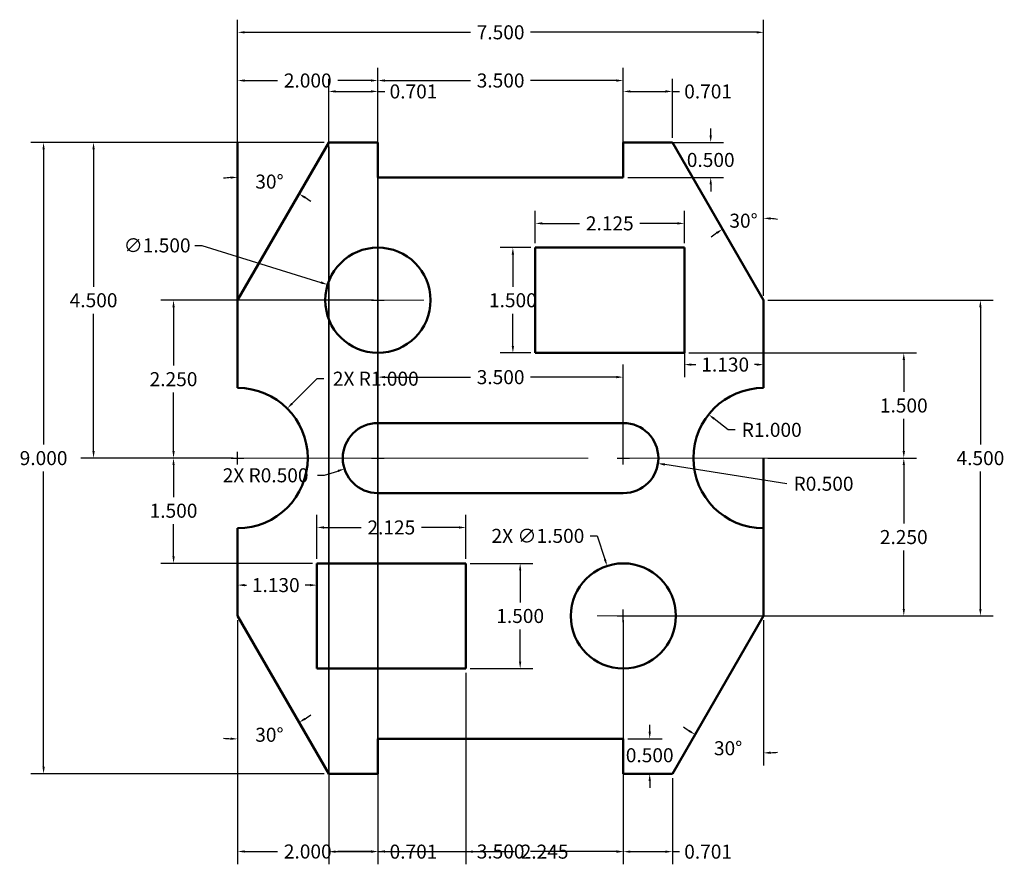
# Model space of a CAD drawing. Units: inches. Extents: x 273.9 to 287.9, y 92.7 to 104.7.
import ezdxf

# ---------------------------------------------------------------- set-up
doc = ezdxf.new("R2010")
doc.units = ezdxf.units.IN
doc.header["$MEASUREMENT"] = 0
doc.linetypes.add('CENTER', pattern=[50.8, 31.75, -6.35, 6.35, -6.35])
for name, color, linetype, lineweight in [('M-CNTR', 114, 'CENTER', 18), ('M-DIMS', 2, 'Continuous', 25), ('M-OUTL', 7, 'Continuous', 50)]:
    doc.layers.add(name, color=color, linetype=linetype, lineweight=lineweight)
doc.styles.get("Standard").update_dxf_attribs({"font": 'arial.ttf'})
doc.dimstyles.get("Standard").update_dxf_attribs({"dimtxt": 0.2, "dimasz": 0.1, "dimexe": 0.18, "dimexo": 0.0625, "dimgap": 0.09, "dimtad": 0, "dimtih": 1, "dimtoh": 1, "dimdec": 3, "dimzin": 0, "dimdsep": 46, "dimtxsty": 'Standard', "dimcen": 0.09, "dimclrd": 1, "dimclre": 1, "dimclrt": 256, "dimadec": 0, "dimazin": 0, "dimtfac": 1, "dimtdec": 3, "dimtofl": 0, "dimtmove": 0, "dimatfit": 3, "dimfxl": 1, "dimtfillclr": 1, "dimtolj": 1, "dimtzin": 0, "dimarcsym": 0})

# ---------------------------------------------------------------- blocks, each defined once
blk = doc.blocks.new('*D1')
at = {"layer": 'Defpoints', "color": 0, "transparency": 16777216}
for p in [(278.973, 94.472), (282.473, 94.472), (282.473, 92.865)]:
    blk.add_point(p, dxfattribs=at)
at = {"layer": 'M-DIMS', "color": 0, "lineweight": -2, "transparency": 16777216}
for p, q in [((278.973, 94.41), (278.973, 92.685)), ((282.473, 94.41), (282.473, 92.685)), ((279.073, 92.865), (280.296, 92.865)), ((282.373, 92.865), (281.15, 92.865))]:
    blk.add_line(p, q, dxfattribs=at)
at = {"layer": 'M-DIMS', "color": 0, "transparency": 16777216}
for points in [[(279.073, 92.882), (279.073, 92.849), (278.973, 92.865)], [(282.373, 92.882), (282.373, 92.849), (282.473, 92.865)]]:
    blk.add_solid(points, dxfattribs=at)
at = {"layer": 'M-DIMS', "color": 0, "transparency": 16777216, "insert": (280.723, 92.865), "char_height": 0.2, "attachment_point": 5}
blk.add_mtext('\\A1;3.500', dxfattribs=at)
blk = doc.blocks.new('*D2')
at = {"layer": 'Defpoints', "color": 0, "transparency": 16777216}
for p in [(282.473, 94.472), (282.473, 93.972), (282.849, 93.972)]:
    blk.add_point(p, dxfattribs=at)
at = {"layer": 'M-DIMS', "color": 0, "lineweight": -2, "transparency": 16777216}
for p, q in [((282.849, 94.572), (282.849, 94.672)), ((282.535, 94.472), (283.029, 94.472)), ((282.535, 93.972), (283.029, 93.972)), ((282.849, 93.872), (282.849, 93.772))]:
    blk.add_line(p, q, dxfattribs=at)
at = {"layer": 'M-DIMS', "color": 0, "transparency": 16777216}
for points in [[(282.833, 94.572), (282.866, 94.572), (282.849, 94.472)], [(282.833, 93.872), (282.866, 93.872), (282.849, 93.972)]]:
    blk.add_solid(points, dxfattribs=at)
at = {"layer": 'M-DIMS', "color": 0, "transparency": 16777216, "insert": (282.849, 94.237), "char_height": 0.2, "attachment_point": 5}
blk.add_mtext('\\A1;0.500', dxfattribs=at)
blk = doc.blocks.new('*D3')
at = {"layer": 'Defpoints', "color": 0, "transparency": 16777216}
for p in [(282.473, 103.854), (278.973, 102.472), (282.473, 102.472)]:
    blk.add_point(p, dxfattribs=at)
at = {"layer": 'M-DIMS', "color": 0, "lineweight": -2, "transparency": 16777216}
for p, q in [((278.973, 102.535), (278.973, 104.034)), ((282.473, 102.535), (282.473, 104.034)), ((279.073, 103.854), (280.296, 103.854)), ((282.373, 103.854), (281.15, 103.854))]:
    blk.add_line(p, q, dxfattribs=at)
at = {"layer": 'M-DIMS', "color": 0, "transparency": 16777216}
for points in [[(279.073, 103.87), (279.073, 103.837), (278.973, 103.854)], [(282.373, 103.87), (282.373, 103.837), (282.473, 103.854)]]:
    blk.add_solid(points, dxfattribs=at)
at = {"layer": 'M-DIMS', "color": 0, "transparency": 16777216, "insert": (280.723, 103.854), "char_height": 0.2, "attachment_point": 5}
blk.add_mtext('\\A1;3.500', dxfattribs=at)
blk = doc.blocks.new('*D4')
at = {"layer": 'Defpoints', "color": 0, "transparency": 16777216}
for p in [(282.473, 99.626), (278.973, 98.472), (282.473, 98.472)]:
    blk.add_point(p, dxfattribs=at)
at = {"layer": 'M-DIMS', "color": 0, "lineweight": -2, "transparency": 16777216}
for p, q in [((278.973, 98.535), (278.973, 99.806)), ((282.473, 98.535), (282.473, 99.806)), ((279.073, 99.626), (280.296, 99.626)), ((282.373, 99.626), (281.15, 99.626))]:
    blk.add_line(p, q, dxfattribs=at)
at = {"layer": 'M-DIMS', "color": 0, "transparency": 16777216}
for points in [[(279.073, 99.643), (279.073, 99.61), (278.973, 99.626)], [(282.373, 99.643), (282.373, 99.61), (282.473, 99.626)]]:
    blk.add_solid(points, dxfattribs=at)
at = {"layer": 'M-DIMS', "color": 0, "transparency": 16777216, "insert": (280.723, 99.626), "char_height": 0.2, "attachment_point": 5}
blk.add_mtext('\\A1;3.500', dxfattribs=at)
blk = doc.blocks.new('*D5')
at = {"layer": 'Defpoints', "color": 0, "transparency": 16777216}
for p in [(280.228, 96.972), (281.002, 96.972), (280.228, 95.472)]:
    blk.add_point(p, dxfattribs=at)
at = {"layer": 'M-DIMS', "color": 0, "lineweight": -2, "transparency": 16777216}
for p, q in [((280.29, 96.972), (281.182, 96.972)), ((281.002, 96.872), (281.002, 96.415)), ((281.002, 95.572), (281.002, 96.03)), ((280.29, 95.472), (281.182, 95.472))]:
    blk.add_line(p, q, dxfattribs=at)
at = {"layer": 'M-DIMS', "color": 0, "transparency": 16777216}
for points in [[(280.985, 96.872), (281.018, 96.872), (281.002, 96.972)], [(280.985, 95.572), (281.018, 95.572), (281.002, 95.472)]]:
    blk.add_solid(points, dxfattribs=at)
at = {"layer": 'M-DIMS', "color": 0, "transparency": 16777216, "insert": (281.002, 96.222), "char_height": 0.2, "attachment_point": 5}
blk.add_mtext('\\A1;1.500', dxfattribs=at)
blk = doc.blocks.new('*D6')
at = {"layer": 'Defpoints', "color": 0, "transparency": 16777216}
for p in [(278.103, 97.484), (278.103, 96.972), (280.228, 96.972)]:
    blk.add_point(p, dxfattribs=at)
at = {"layer": 'M-DIMS', "color": 0, "lineweight": -2, "transparency": 16777216}
for p, q in [((278.103, 97.035), (278.103, 97.664)), ((280.228, 97.035), (280.228, 97.664)), ((278.203, 97.484), (278.735, 97.484)), ((280.128, 97.484), (279.595, 97.484))]:
    blk.add_line(p, q, dxfattribs=at)
at = {"layer": 'M-DIMS', "color": 0, "transparency": 16777216}
for points in [[(278.203, 97.5), (278.203, 97.467), (278.103, 97.484)], [(280.128, 97.5), (280.128, 97.467), (280.228, 97.484)]]:
    blk.add_solid(points, dxfattribs=at)
at = {"layer": 'M-DIMS', "color": 0, "transparency": 16777216, "insert": (279.165, 97.484), "char_height": 0.2, "attachment_point": 5}
blk.add_mtext('\\A1;2.125', dxfattribs=at)
blk = doc.blocks.new('*D7')
at = {"layer": 'Defpoints', "color": 0, "transparency": 16777216}
for p in [(276.973, 97.045), (276.973, 96.662), (278.103, 96.275)]:
    blk.add_point(p, dxfattribs=at)
at = {"layer": 'M-DIMS', "color": 0, "lineweight": -2, "transparency": 16777216}
for p, q in [((276.973, 96.982), (276.973, 96.482)), ((278.103, 96.337), (278.103, 96.842)), ((277.073, 96.662), (277.099, 96.662)), ((278.003, 96.662), (277.935, 96.662))]:
    blk.add_line(p, q, dxfattribs=at)
at = {"layer": 'M-DIMS', "color": 0, "transparency": 16777216}
for points in [[(277.073, 96.678), (277.073, 96.645), (276.973, 96.662)], [(278.003, 96.678), (278.003, 96.645), (278.103, 96.662)]]:
    blk.add_solid(points, dxfattribs=at)
at = {"layer": 'M-DIMS', "color": 0, "transparency": 16777216, "insert": (277.517, 96.662), "char_height": 0.2, "attachment_point": 5}
blk.add_mtext('\\A1;1.130', dxfattribs=at)
blk = doc.blocks.new('*D8')
at = {"layer": 'Defpoints', "color": 0, "transparency": 16777216}
for p in [(276.973, 98.472), (276.059, 96.972), (278.103, 96.972)]:
    blk.add_point(p, dxfattribs=at)
at = {"layer": 'M-DIMS', "color": 0, "lineweight": -2, "transparency": 16777216}
for p, q in [((276.91, 98.472), (275.879, 98.472)), ((276.059, 98.372), (276.059, 97.915)), ((276.059, 97.072), (276.059, 97.53)), ((278.04, 96.972), (275.879, 96.972))]:
    blk.add_line(p, q, dxfattribs=at)
at = {"layer": 'M-DIMS', "color": 0, "transparency": 16777216}
for points in [[(276.043, 98.372), (276.076, 98.372), (276.059, 98.472)], [(276.043, 97.072), (276.076, 97.072), (276.059, 96.972)]]:
    blk.add_solid(points, dxfattribs=at)
at = {"layer": 'M-DIMS', "color": 0, "transparency": 16777216, "insert": (276.059, 97.722), "char_height": 0.2, "attachment_point": 5}
blk.add_mtext('\\A1;1.500', dxfattribs=at)
blk = doc.blocks.new('*D9')
at = {"layer": 'Defpoints', "color": 0, "transparency": 16777216}
for p in [(278.973, 100.722), (276.059, 98.472), (276.973, 98.472)]:
    blk.add_point(p, dxfattribs=at)
at = {"layer": 'M-DIMS', "color": 0, "lineweight": -2, "transparency": 16777216}
for p, q in [((278.91, 100.722), (275.879, 100.722)), ((276.059, 100.622), (276.059, 99.79)), ((276.059, 98.572), (276.059, 99.405)), ((276.91, 98.472), (275.879, 98.472))]:
    blk.add_line(p, q, dxfattribs=at)
at = {"layer": 'M-DIMS', "color": 0, "transparency": 16777216}
for points in [[(276.043, 100.622), (276.076, 100.622), (276.059, 100.722)], [(276.043, 98.572), (276.076, 98.572), (276.059, 98.472)]]:
    blk.add_solid(points, dxfattribs=at)
at = {"layer": 'M-DIMS', "color": 0, "transparency": 16777216, "insert": (276.059, 99.597), "char_height": 0.2, "attachment_point": 5}
blk.add_mtext('\\A1;2.250', dxfattribs=at)
blk = doc.blocks.new('*D10')
at = {"layer": 'Defpoints', "color": 0, "transparency": 16777216}
for p in [(281.218, 101.818), (281.218, 101.472), (283.343, 101.472)]:
    blk.add_point(p, dxfattribs=at)
at = {"layer": 'M-DIMS', "color": 0, "lineweight": -2, "transparency": 16777216}
for p, q in [((281.218, 101.535), (281.218, 101.998)), ((283.343, 101.535), (283.343, 101.998)), ((281.318, 101.818), (281.85, 101.818)), ((283.243, 101.818), (282.71, 101.818))]:
    blk.add_line(p, q, dxfattribs=at)
at = {"layer": 'M-DIMS', "color": 0, "transparency": 16777216}
for points in [[(281.318, 101.834), (281.318, 101.801), (281.218, 101.818)], [(283.243, 101.834), (283.243, 101.801), (283.343, 101.818)]]:
    blk.add_solid(points, dxfattribs=at)
at = {"layer": 'M-DIMS', "color": 0, "transparency": 16777216, "insert": (282.28, 101.818), "char_height": 0.2, "attachment_point": 5}
blk.add_mtext('\\A1;2.125', dxfattribs=at)
blk = doc.blocks.new('*D11')
at = {"layer": 'Defpoints', "color": 0, "transparency": 16777216}
for p in [(281.218, 101.472), (280.898, 99.972), (281.218, 99.972)]:
    blk.add_point(p, dxfattribs=at)
at = {"layer": 'M-DIMS', "color": 0, "lineweight": -2, "transparency": 16777216}
for p, q in [((281.155, 101.472), (280.718, 101.472)), ((280.898, 101.372), (280.898, 100.915)), ((280.898, 100.072), (280.898, 100.53)), ((281.155, 99.972), (280.718, 99.972))]:
    blk.add_line(p, q, dxfattribs=at)
at = {"layer": 'M-DIMS', "color": 0, "transparency": 16777216}
for points in [[(280.881, 101.372), (280.915, 101.372), (280.898, 101.472)], [(280.881, 100.072), (280.915, 100.072), (280.898, 99.972)]]:
    blk.add_solid(points, dxfattribs=at)
at = {"layer": 'M-DIMS', "color": 0, "transparency": 16777216, "insert": (280.898, 100.722), "char_height": 0.2, "attachment_point": 5}
blk.add_mtext('\\A1;1.500', dxfattribs=at)
blk = doc.blocks.new('*D12')
at = {"layer": 'Defpoints', "color": 0, "transparency": 16777216}
for p in [(283.343, 100.363), (284.473, 99.805), (284.473, 99.79)]:
    blk.add_point(p, dxfattribs=at)
at = {"layer": 'M-DIMS', "color": 0, "lineweight": -2, "transparency": 16777216}
for p, q in [((283.343, 100.3), (283.343, 99.625)), ((284.473, 99.853), (284.473, 99.985)), ((283.443, 99.805), (283.508, 99.805)), ((284.373, 99.805), (284.343, 99.805))]:
    blk.add_line(p, q, dxfattribs=at)
at = {"layer": 'M-DIMS', "color": 0, "transparency": 16777216}
for points in [[(283.443, 99.821), (283.443, 99.788), (283.343, 99.805)], [(284.373, 99.821), (284.373, 99.788), (284.473, 99.805)]]:
    blk.add_solid(points, dxfattribs=at)
at = {"layer": 'M-DIMS', "color": 0, "transparency": 16777216, "insert": (283.926, 99.805), "char_height": 0.2, "attachment_point": 5}
blk.add_mtext('\\A1;1.130', dxfattribs=at)
blk = doc.blocks.new('*D13')
at = {"layer": 'Defpoints', "color": 0, "transparency": 16777216}
for p in [(283.174, 102.972), (284.073, 101.821), (284.473, 100.722), (284.473, 100.722), (284.473, 99.472)]:
    blk.add_point(p, dxfattribs=at)
at = {"layer": 'M-DIMS', "color": 0, "lineweight": -2, "transparency": 16777216}
blk.add_line((284.473, 100.785), (284.473, 102.071), dxfattribs=at)
for start, end in [(80.1925, 85.0963), (124.9037, 129.8075)]:
    blk.add_arc((284.473, 100.722), 1.169, start, end, dxfattribs=at)
at = {"layer": 'M-DIMS', "color": 0, "transparency": 16777216}
for points in [[(284.572, 101.87), (284.573, 101.904), (284.473, 101.891)], [(283.795, 101.695), (283.813, 101.667), (283.888, 101.735)]]:
    blk.add_solid(points, dxfattribs=at)
at = {"layer": 'M-DIMS', "color": 0, "transparency": 16777216, "insert": (284.187, 101.856), "char_height": 0.2, "attachment_point": 5}
blk.add_mtext('\\A1;30°', dxfattribs=at)
blk = doc.blocks.new('*D14')
at = {"layer": 'Defpoints', "color": 0, "transparency": 16777216}
for p in [(276.973, 96.222), (276.973, 96.222), (277.277, 94.496), (276.973, 94.41), (278.272, 93.972)]:
    blk.add_point(p, dxfattribs=at)
at = {"layer": 'M-DIMS', "color": 0, "lineweight": -2, "transparency": 16777216}
for start, end in [(303.2689, 306.5377), (263.4623, 266.7311)]:
    blk.add_arc((276.973, 96.222), 1.753, start, end, dxfattribs=at)
at = {"layer": 'M-DIMS', "color": 0, "transparency": 16777216}
for points in [[(277.943, 94.743), (277.925, 94.771), (277.849, 94.704)], [(276.873, 94.489), (276.872, 94.456), (276.973, 94.469)]]:
    blk.add_solid(points, dxfattribs=at)
at = {"layer": 'M-DIMS', "color": 0, "transparency": 16777216, "insert": (277.426, 94.529), "char_height": 0.2, "attachment_point": 5}
blk.add_mtext('\\A1;30°', dxfattribs=at)
blk = doc.blocks.new('*D15')
at = {"layer": 'Defpoints', "color": 0, "transparency": 16777216}
for p in [(276.973, 96.222), (278.973, 93.972), (278.973, 92.865)]:
    blk.add_point(p, dxfattribs=at)
at = {"layer": 'M-DIMS', "color": 0, "lineweight": -2, "transparency": 16777216}
for p, q in [((276.973, 96.16), (276.973, 92.685)), ((278.973, 93.91), (278.973, 92.685)), ((277.073, 92.865), (277.544, 92.865)), ((278.873, 92.865), (278.401, 92.865))]:
    blk.add_line(p, q, dxfattribs=at)
at = {"layer": 'M-DIMS', "color": 0, "transparency": 16777216}
for points in [[(277.073, 92.882), (277.073, 92.849), (276.973, 92.865)], [(278.873, 92.882), (278.873, 92.849), (278.973, 92.865)]]:
    blk.add_solid(points, dxfattribs=at)
at = {"layer": 'M-DIMS', "color": 0, "transparency": 16777216, "insert": (277.973, 92.865), "char_height": 0.2, "attachment_point": 5}
blk.add_mtext('\\A1;2.000', dxfattribs=at)
blk = doc.blocks.new('*D16')
at = {"layer": 'Defpoints', "color": 0, "transparency": 16777216}
for p in [(283.69, 99.094), (284.473, 98.472)]:
    blk.add_point(p, dxfattribs=at)
at = {"layer": 'M-DIMS', "color": 0, "lineweight": -2, "transparency": 16777216}
for p, q in [((283.966, 98.875), (283.768, 99.032)), ((284.066, 98.875), (283.966, 98.875))]:
    blk.add_line(p, q, dxfattribs=at)
at = {"layer": 'M-DIMS', "color": 0, "transparency": 16777216}
blk.add_solid([(283.778, 99.045), (283.758, 99.019), (283.69, 99.094)], dxfattribs=at)
at = {"layer": 'M-DIMS', "color": 0, "transparency": 16777216, "insert": (284.589, 98.875), "char_height": 0.2, "attachment_point": 5}
blk.add_mtext('\\A1;R1.000', dxfattribs=at)
blk = doc.blocks.new('*D17')
at = {"layer": 'Defpoints', "color": 0, "transparency": 16777216}
for p in [(282.473, 98.472), (282.967, 98.395)]:
    blk.add_point(p, dxfattribs=at)
at = {"layer": 'M-DIMS', "color": 0, "lineweight": -2, "transparency": 16777216}
for p, q in [((282.473, 98.382), (282.473, 98.562)), ((282.383, 98.472), (282.563, 98.472)), ((284.805, 98.107), (283.065, 98.38))]:
    blk.add_line(p, q, dxfattribs=at)
at = {"layer": 'M-DIMS', "color": 0, "transparency": 16777216}
blk.add_solid([(283.068, 98.396), (283.063, 98.363), (282.967, 98.395)], dxfattribs=at)
at = {"layer": 'M-DIMS', "color": 0, "transparency": 16777216, "insert": (285.328, 98.107), "char_height": 0.2, "attachment_point": 5}
blk.add_mtext('\\A1;R0.500', dxfattribs=at)
blk = doc.blocks.new('*D18')
at = {"layer": 'Defpoints', "color": 0, "transparency": 16777216}
for p in [(284.473, 98.472), (282.473, 96.222), (286.472, 96.222)]:
    blk.add_point(p, dxfattribs=at)
at = {"layer": 'M-DIMS', "color": 0, "lineweight": -2, "transparency": 16777216}
for p, q in [((284.535, 98.472), (286.652, 98.472)), ((286.472, 98.372), (286.472, 97.54)), ((286.472, 96.322), (286.472, 97.155)), ((282.535, 96.222), (286.652, 96.222))]:
    blk.add_line(p, q, dxfattribs=at)
at = {"layer": 'M-DIMS', "color": 0, "transparency": 16777216}
for points in [[(286.456, 98.372), (286.489, 98.372), (286.472, 98.472)], [(286.456, 96.322), (286.489, 96.322), (286.472, 96.222)]]:
    blk.add_solid(points, dxfattribs=at)
at = {"layer": 'M-DIMS', "color": 0, "transparency": 16777216, "insert": (286.472, 97.347), "char_height": 0.2, "attachment_point": 5}
blk.add_mtext('\\A1;2.250', dxfattribs=at)
blk = doc.blocks.new('*D19')
at = {"layer": 'Defpoints', "color": 0, "transparency": 16777216}
for p in [(283.343, 99.972), (286.472, 99.972), (284.473, 98.472)]:
    blk.add_point(p, dxfattribs=at)
at = {"layer": 'M-DIMS', "color": 0, "lineweight": -2, "transparency": 16777216}
for p, q in [((283.405, 99.972), (286.652, 99.972)), ((286.472, 99.872), (286.472, 99.415)), ((286.472, 98.572), (286.472, 99.03)), ((284.535, 98.472), (286.652, 98.472))]:
    blk.add_line(p, q, dxfattribs=at)
at = {"layer": 'M-DIMS', "color": 0, "transparency": 16777216}
for points in [[(286.456, 99.872), (286.489, 99.872), (286.472, 99.972)], [(286.456, 98.572), (286.489, 98.572), (286.472, 98.472)]]:
    blk.add_solid(points, dxfattribs=at)
at = {"layer": 'M-DIMS', "color": 0, "transparency": 16777216, "insert": (286.472, 99.222), "char_height": 0.2, "attachment_point": 5}
blk.add_mtext('\\A1;1.500', dxfattribs=at)
blk = doc.blocks.new('*D20')
at = {"layer": 'Defpoints', "color": 0, "transparency": 16777216}
for p in [(284.473, 100.722), (287.565, 100.722), (284.473, 96.222)]:
    blk.add_point(p, dxfattribs=at)
at = {"layer": 'M-DIMS', "color": 0, "lineweight": -2, "transparency": 16777216}
for p, q in [((284.535, 100.722), (287.745, 100.722)), ((287.565, 100.622), (287.565, 98.665)), ((287.565, 96.322), (287.565, 98.28)), ((284.535, 96.222), (287.745, 96.222))]:
    blk.add_line(p, q, dxfattribs=at)
at = {"layer": 'M-DIMS', "color": 0, "transparency": 16777216}
for points in [[(287.548, 100.622), (287.581, 100.622), (287.565, 100.722)], [(287.548, 96.322), (287.581, 96.322), (287.565, 96.222)]]:
    blk.add_solid(points, dxfattribs=at)
at = {"layer": 'M-DIMS', "color": 0, "transparency": 16777216, "insert": (287.565, 98.472), "char_height": 0.2, "attachment_point": 5}
blk.add_mtext('\\A1;4.500', dxfattribs=at)
blk = doc.blocks.new('*D21')
at = {"layer": 'Defpoints', "color": 0, "transparency": 16777216}
for p in [(276.973, 102.972), (278.272, 102.972), (277.277, 102.447), (276.973, 100.722), (276.973, 99.472)]:
    blk.add_point(p, dxfattribs=at)
at = {"layer": 'M-DIMS', "color": 0, "lineweight": -2, "transparency": 16777216}
for start, end in [(93.2724, 96.5449), (53.4551, 56.7276)]:
    blk.add_arc((276.973, 100.722), 1.751, start, end, dxfattribs=at)
at = {"layer": 'M-DIMS', "color": 0, "transparency": 16777216}
for points in [[(276.872, 102.487), (276.873, 102.454), (276.973, 102.474)], [(277.925, 102.172), (277.942, 102.201), (277.848, 102.239)]]:
    blk.add_solid(points, dxfattribs=at)
at = {"layer": 'M-DIMS', "color": 0, "transparency": 16777216, "insert": (277.427, 102.413), "char_height": 0.2, "attachment_point": 5}
blk.add_mtext('\\A1;30°', dxfattribs=at)
blk = doc.blocks.new('*D22')
at = {"layer": 'Defpoints', "color": 0, "transparency": 16777216}
for p in [(284.473, 104.541), (276.973, 100.722), (284.473, 100.722)]:
    blk.add_point(p, dxfattribs=at)
at = {"layer": 'M-DIMS', "color": 0, "lineweight": -2, "transparency": 16777216}
for p, q in [((276.973, 100.785), (276.973, 104.721)), ((284.473, 100.785), (284.473, 104.721)), ((277.073, 104.541), (280.296, 104.541)), ((284.373, 104.541), (281.149, 104.541))]:
    blk.add_line(p, q, dxfattribs=at)
at = {"layer": 'M-DIMS', "color": 0, "transparency": 16777216}
for points in [[(277.073, 104.557), (277.073, 104.524), (276.973, 104.541)], [(284.373, 104.557), (284.373, 104.524), (284.473, 104.541)]]:
    blk.add_solid(points, dxfattribs=at)
at = {"layer": 'M-DIMS', "color": 0, "transparency": 16777216, "insert": (280.723, 104.541), "char_height": 0.2, "attachment_point": 5}
blk.add_mtext('\\A1;7.500', dxfattribs=at)
blk = doc.blocks.new('*D23')
at = {"layer": 'Defpoints', "color": 0, "transparency": 16777216}
for p in [(278.973, 103.854), (278.973, 102.972), (276.973, 100.722)]:
    blk.add_point(p, dxfattribs=at)
at = {"layer": 'M-DIMS', "color": 0, "lineweight": -2, "transparency": 16777216}
for p, q in [((276.973, 100.785), (276.973, 104.034)), ((278.973, 103.035), (278.973, 104.034)), ((277.073, 103.854), (277.544, 103.854)), ((278.873, 103.854), (278.401, 103.854))]:
    blk.add_line(p, q, dxfattribs=at)
at = {"layer": 'M-DIMS', "color": 0, "transparency": 16777216}
for points in [[(277.073, 103.87), (277.073, 103.837), (276.973, 103.854)], [(278.873, 103.87), (278.873, 103.837), (278.973, 103.854)]]:
    blk.add_solid(points, dxfattribs=at)
at = {"layer": 'M-DIMS', "color": 0, "transparency": 16777216, "insert": (277.973, 103.854), "char_height": 0.2, "attachment_point": 5}
blk.add_mtext('\\A1;2.000', dxfattribs=at)
blk = doc.blocks.new('*D24')
at = {"layer": 'Defpoints', "color": 0, "transparency": 16777216}
for p in [(282.473, 102.972), (283.719, 102.972), (282.473, 102.472)]:
    blk.add_point(p, dxfattribs=at)
at = {"layer": 'M-DIMS', "color": 0, "lineweight": -2, "transparency": 16777216}
for p, q in [((283.719, 103.072), (283.719, 103.172)), ((282.535, 102.972), (283.899, 102.972)), ((282.535, 102.472), (283.899, 102.472)), ((283.719, 102.372), (283.719, 102.272))]:
    blk.add_line(p, q, dxfattribs=at)
at = {"layer": 'M-DIMS', "color": 0, "transparency": 16777216}
for points in [[(283.702, 103.072), (283.736, 103.072), (283.719, 102.972)], [(283.702, 102.372), (283.736, 102.372), (283.719, 102.472)]]:
    blk.add_solid(points, dxfattribs=at)
at = {"layer": 'M-DIMS', "color": 0, "transparency": 16777216, "insert": (283.719, 102.722), "char_height": 0.2, "attachment_point": 5}
blk.add_mtext('\\A1;0.500', dxfattribs=at)
blk = doc.blocks.new('*D25')
at = {"layer": 'Defpoints', "color": 0, "transparency": 16777216}
for p in [(278.256, 100.945), (279.689, 100.5)]:
    blk.add_point(p, dxfattribs=at)
at = {"layer": 'M-DIMS', "color": 0, "lineweight": -2, "transparency": 16777216}
for p, q in [((276.361, 101.504), (276.461, 101.504)), ((276.461, 101.504), (278.161, 100.975)), ((278.973, 100.632), (278.973, 100.812)), ((278.883, 100.722), (279.063, 100.722))]:
    blk.add_line(p, q, dxfattribs=at)
at = {"layer": 'M-DIMS', "color": 0, "transparency": 16777216}
blk.add_solid([(278.166, 100.991), (278.156, 100.959), (278.256, 100.945)], dxfattribs=at)
at = {"layer": 'M-DIMS', "color": 0, "transparency": 16777216, "insert": (275.825, 101.504), "char_height": 0.2, "attachment_point": 5}
blk.add_mtext('\\A1;∅1.500', dxfattribs=at)
blk = doc.blocks.new('*D26')
at = {"layer": 'Defpoints', "color": 0, "transparency": 16777216}
for p in [(278.272, 102.972), (274.206, 93.972), (278.272, 93.972)]:
    blk.add_point(p, dxfattribs=at)
at = {"layer": 'M-DIMS', "color": 0, "lineweight": -2, "transparency": 16777216}
for p, q in [((278.209, 102.972), (274.026, 102.972)), ((274.206, 102.872), (274.206, 98.665)), ((274.206, 94.072), (274.206, 98.28)), ((278.209, 93.972), (274.026, 93.972))]:
    blk.add_line(p, q, dxfattribs=at)
at = {"layer": 'M-DIMS', "color": 0, "transparency": 16777216}
for points in [[(274.19, 102.872), (274.223, 102.872), (274.206, 102.972)], [(274.19, 94.072), (274.223, 94.072), (274.206, 93.972)]]:
    blk.add_solid(points, dxfattribs=at)
at = {"layer": 'M-DIMS', "color": 0, "transparency": 16777216, "insert": (274.206, 98.472), "char_height": 0.2, "attachment_point": 5}
blk.add_mtext('\\A1;9.000', dxfattribs=at)
blk = doc.blocks.new('*D27')
at = {"layer": 'Defpoints', "color": 0, "transparency": 16777216}
for p in [(278.272, 102.972), (274.919, 98.472), (276.973, 98.472)]:
    blk.add_point(p, dxfattribs=at)
at = {"layer": 'M-DIMS', "color": 0, "lineweight": -2, "transparency": 16777216}
for p, q in [((278.209, 102.972), (274.739, 102.972)), ((274.919, 102.872), (274.919, 100.915)), ((274.919, 98.572), (274.919, 100.53)), ((276.91, 98.472), (274.739, 98.472))]:
    blk.add_line(p, q, dxfattribs=at)
at = {"layer": 'M-DIMS', "color": 0, "transparency": 16777216}
for points in [[(274.902, 102.872), (274.935, 102.872), (274.919, 102.972)], [(274.902, 98.572), (274.935, 98.572), (274.919, 98.472)]]:
    blk.add_solid(points, dxfattribs=at)
at = {"layer": 'M-DIMS', "color": 0, "transparency": 16777216, "insert": (274.919, 100.722), "char_height": 0.2, "attachment_point": 5}
blk.add_mtext('\\A1;4.500', dxfattribs=at)
blk = doc.blocks.new('*D28')
at = {"layer": 'Defpoints', "color": 0, "transparency": 16777216}
for p in [(284.473, 98.472), (284.473, 96.222), (284.473, 96.222), (283.805, 94.388), (283.174, 93.972)]:
    blk.add_point(p, dxfattribs=at)
at = {"layer": 'M-DIMS', "color": 0, "lineweight": -2, "transparency": 16777216}
blk.add_line((284.473, 96.16), (284.473, 94.09), dxfattribs=at)
for start, end in [(234.1288, 237.0644), (272.9356, 275.8712)]:
    blk.add_arc((284.473, 96.222), 1.952, start, end, dxfattribs=at)
at = {"layer": 'M-DIMS', "color": 0, "transparency": 16777216}
for points in [[(283.42, 94.598), (283.403, 94.57), (283.497, 94.532)], [(284.573, 94.256), (284.572, 94.29), (284.473, 94.27)]]:
    blk.add_solid(points, dxfattribs=at)
at = {"layer": 'M-DIMS', "color": 0, "transparency": 16777216, "insert": (283.967, 94.337), "char_height": 0.2, "attachment_point": 5}
blk.add_mtext('\\A1;30°', dxfattribs=at)
blk = doc.blocks.new('CUTOUT-RECT-2.125X1.50')
for p, q in [((0, 1.5), (0, 0)), ((2.125, 1.5), (0, 1.5)), ((2.125, 0), (2.125, 1.5)), ((0, 0), (2.125, 0))]:
    blk.add_line(p, q)
blk = doc.blocks.new('HOLE-DIA-1.50')
blk.add_circle((0.75, 0.75), 0.75)
blk = doc.blocks.new('*D31')
at = {"layer": 'Defpoints', "color": 0, "transparency": 16777216}
for p in [(278.973, 103.698), (278.272, 93.972), (278.973, 93.972)]:
    blk.add_point(p, dxfattribs=at)
at = {"layer": 'M-DIMS', "color": 1, "lineweight": -2, "transparency": 16777216}
for p, q in [((278.272, 94.035), (278.272, 103.878)), ((278.973, 94.035), (278.973, 103.878)), ((278.372, 103.698), (278.873, 103.698)), ((278.973, 103.698), (279.073, 103.698))]:
    blk.add_line(p, q, dxfattribs=at)
at = {"layer": 'M-DIMS', "color": 1, "transparency": 16777216}
for points in [[(278.372, 103.715), (278.372, 103.682), (278.272, 103.698)], [(278.873, 103.715), (278.873, 103.682), (278.973, 103.698)]]:
    blk.add_solid(points, dxfattribs=at)
at = {"layer": 'M-DIMS', "transparency": 16777216, "insert": (279.481, 103.698), "char_height": 0.2, "attachment_point": 5}
blk.add_mtext('\\A1;0.701', dxfattribs=at)
blk = doc.blocks.new('*D32')
at = {"layer": 'Defpoints', "color": 0, "transparency": 16777216}
for p in [(282.473, 96.222), (280.228, 95.472), (282.473, 92.863)]:
    blk.add_point(p, dxfattribs=at)
at = {"layer": 'M-DIMS', "color": 1, "lineweight": -2, "transparency": 16777216}
for p, q in [((282.473, 96.16), (282.473, 92.683)), ((280.228, 95.41), (280.228, 92.683)), ((280.328, 92.863), (280.92, 92.863)), ((282.373, 92.863), (281.78, 92.863))]:
    blk.add_line(p, q, dxfattribs=at)
at = {"layer": 'M-DIMS', "color": 1, "transparency": 16777216}
for points in [[(280.328, 92.879), (280.328, 92.846), (280.228, 92.863)], [(282.373, 92.879), (282.373, 92.846), (282.473, 92.863)]]:
    blk.add_solid(points, dxfattribs=at)
at = {"layer": 'M-DIMS', "transparency": 16777216, "insert": (281.35, 92.863), "char_height": 0.2, "attachment_point": 5}
blk.add_mtext('\\A1;2.245', dxfattribs=at)
blk = doc.blocks.new('*D33')
at = {"layer": 'Defpoints', "color": 0, "transparency": 16777216}
for p in [(278.272, 102.972), (278.973, 102.972), (278.973, 92.863)]:
    blk.add_point(p, dxfattribs=at)
at = {"layer": 'M-DIMS', "color": 1, "lineweight": -2, "transparency": 16777216}
for p, q in [((278.272, 102.91), (278.272, 92.683)), ((278.973, 102.91), (278.973, 92.683)), ((278.372, 92.863), (278.873, 92.863)), ((278.973, 92.863), (279.073, 92.863))]:
    blk.add_line(p, q, dxfattribs=at)
at = {"layer": 'M-DIMS', "color": 1, "transparency": 16777216}
for points in [[(278.372, 92.879), (278.372, 92.846), (278.272, 92.863)], [(278.873, 92.879), (278.873, 92.846), (278.973, 92.863)]]:
    blk.add_solid(points, dxfattribs=at)
at = {"layer": 'M-DIMS', "transparency": 16777216, "insert": (279.481, 92.863), "char_height": 0.2, "attachment_point": 5}
blk.add_mtext('\\A1;0.701', dxfattribs=at)
blk = doc.blocks.new('*D34')
at = {"layer": 'Defpoints', "color": 0, "transparency": 16777216}
for p in [(283.174, 103.698), (282.473, 102.972), (283.174, 102.972)]:
    blk.add_point(p, dxfattribs=at)
at = {"layer": 'M-DIMS', "color": 1, "lineweight": -2, "transparency": 16777216}
for p, q in [((282.473, 103.035), (282.473, 103.878)), ((283.174, 103.035), (283.174, 103.878)), ((282.573, 103.698), (283.074, 103.698)), ((283.174, 103.698), (283.274, 103.698))]:
    blk.add_line(p, q, dxfattribs=at)
at = {"layer": 'M-DIMS', "color": 1, "transparency": 16777216}
for points in [[(282.573, 103.715), (282.573, 103.682), (282.473, 103.698)], [(283.074, 103.715), (283.074, 103.682), (283.174, 103.698)]]:
    blk.add_solid(points, dxfattribs=at)
at = {"layer": 'M-DIMS', "transparency": 16777216, "insert": (283.682, 103.698), "char_height": 0.2, "attachment_point": 5}
blk.add_mtext('\\A1;0.701', dxfattribs=at)
blk = doc.blocks.new('*D35')
at = {"layer": 'Defpoints', "color": 0, "transparency": 16777216}
for p in [(282.473, 93.972), (283.174, 93.972), (283.174, 92.863)]:
    blk.add_point(p, dxfattribs=at)
at = {"layer": 'M-DIMS', "color": 1, "lineweight": -2, "transparency": 16777216}
for p, q in [((282.473, 93.91), (282.473, 92.683)), ((283.174, 93.91), (283.174, 92.683)), ((282.573, 92.863), (283.074, 92.863)), ((283.174, 92.863), (283.274, 92.863))]:
    blk.add_line(p, q, dxfattribs=at)
at = {"layer": 'M-DIMS', "color": 1, "transparency": 16777216}
for points in [[(282.573, 92.879), (282.573, 92.846), (282.473, 92.863)], [(283.074, 92.879), (283.074, 92.846), (283.174, 92.863)]]:
    blk.add_solid(points, dxfattribs=at)
at = {"layer": 'M-DIMS', "transparency": 16777216, "insert": (283.682, 92.863), "char_height": 0.2, "attachment_point": 5}
blk.add_mtext('\\A1;0.701', dxfattribs=at)
blk = doc.blocks.new('*D36')
at = {"layer": 'Defpoints', "color": 0, "transparency": 16777216}
for p in [(277.68, 99.18), (276.973, 98.472)]:
    blk.add_point(p, dxfattribs=at)
at = {"layer": 'M-DIMS', "color": 1, "lineweight": -2, "transparency": 16777216}
for p, q in [((278.104, 99.604), (277.75, 99.25)), ((278.204, 99.604), (278.104, 99.604)), ((276.973, 98.382), (276.973, 98.562)), ((276.883, 98.472), (277.063, 98.472))]:
    blk.add_line(p, q, dxfattribs=at)
at = {"layer": 'M-DIMS', "color": 1, "transparency": 16777216}
blk.add_solid([(277.739, 99.262), (277.762, 99.239), (277.68, 99.18)], dxfattribs=at)
at = {"layer": 'M-DIMS', "transparency": 16777216, "insert": (278.943, 99.604), "char_height": 0.2, "attachment_point": 5}
blk.add_mtext('\\A1;2X R1.000', dxfattribs=at)
blk = doc.blocks.new('*D37')
at = {"layer": 'Defpoints', "color": 0, "transparency": 16777216}
for p in [(278.973, 98.472), (278.497, 98.319)]:
    blk.add_point(p, dxfattribs=at)
at = {"layer": 'M-DIMS', "color": 1, "lineweight": -2, "transparency": 16777216}
for p, q in [((278.973, 98.382), (278.973, 98.562)), ((278.883, 98.472), (279.063, 98.472)), ((278.211, 98.227), (278.402, 98.288)), ((278.111, 98.227), (278.211, 98.227))]:
    blk.add_line(p, q, dxfattribs=at)
at = {"layer": 'M-DIMS', "color": 1, "transparency": 16777216}
blk.add_solid([(278.396, 98.304), (278.407, 98.272), (278.497, 98.319)], dxfattribs=at)
at = {"layer": 'M-DIMS', "transparency": 16777216, "insert": (277.372, 98.227), "char_height": 0.2, "attachment_point": 5}
blk.add_mtext('\\A1;2X R0.500', dxfattribs=at)
blk = doc.blocks.new('*D38')
at = {"layer": 'Defpoints', "color": 0, "transparency": 16777216}
for p in [(282.241, 96.936), (282.704, 95.509)]:
    blk.add_point(p, dxfattribs=at)
at = {"layer": 'M-DIMS', "color": 1, "lineweight": -2, "transparency": 16777216}
for p, q in [((282.002, 97.364), (282.102, 97.364)), ((282.102, 97.364), (282.21, 97.031)), ((282.383, 96.222), (282.563, 96.222)), ((282.473, 96.132), (282.473, 96.312))]:
    blk.add_line(p, q, dxfattribs=at)
at = {"layer": 'M-DIMS', "color": 1, "transparency": 16777216}
blk.add_solid([(282.226, 97.036), (282.194, 97.026), (282.241, 96.936)], dxfattribs=at)
at = {"layer": 'M-DIMS', "transparency": 16777216, "insert": (281.255, 97.364), "char_height": 0.2, "attachment_point": 5}
blk.add_mtext('\\A1;2X ∅1.500', dxfattribs=at)

msp = doc.modelspace()

# ---------------------------------------------------------------- linework, layer by layer
at = {"layer": 'M-CNTR'}
for p, q in [((278.9726, 101.4724), (278.9726, 93.5887)), ((276.9726, 100.7224), (279.6282, 100.7224)), ((276.2737, 98.4724), (281.9726, 98.4724)), ((282.4726, 98.4724), (285.2073, 98.4724)), ((284.4726, 96.2224), (282.0977, 96.2224))]:
    msp.add_line(p, q, dxfattribs=at)
at = {"layer": 'M-OUTL'}
for p, q in [((276.9726, 99.4724), (276.9726, 102.9724)), ((276.9726, 100.7224), (278.2716, 102.9724)), ((278.2716, 102.9724), (278.9726, 102.9724)), ((278.9726, 102.9724), (278.9726, 102.4724)), ((282.4726, 102.4724), (282.4726, 102.9724)), ((282.4726, 102.9724), (283.1735, 102.9724)), ((284.4726, 100.7224), (283.1735, 102.9724)), ((278.9726, 102.4724), (282.4726, 102.4724)), ((284.4726, 99.4724), (284.4726, 100.7224)), ((278.9726, 98.9724), (282.4726, 98.9724)), ((284.4726, 98.4724), (284.4726, 96.2224)), ((278.9726, 97.9724), (282.4726, 97.9724)), ((276.9726, 96.2224), (276.9726, 97.4724)), ((276.9726, 96.2224), (278.2716, 93.9724)), ((284.4726, 96.2224), (283.1735, 93.9724)), ((278.9726, 93.9724), (278.9726, 94.4724)), ((278.9726, 94.4724), (282.4726, 94.4724)), ((282.4726, 94.4724), (282.4726, 93.9724)), ((278.9726, 93.9724), (278.2716, 93.9724)), ((282.4726, 93.9724), (283.1735, 93.9724))]:
    msp.add_line(p, q, dxfattribs=at)
for centre, radius, start, end in [((276.9726, 98.4724), 1, 270, 90), ((284.4726, 98.4724), 1, 90, 270), ((278.9726, 98.4724), 0.5, 90, 270), ((282.4726, 98.4724), 0.5, 270, 90)]:
    msp.add_arc(centre, radius, start, end, dxfattribs=at)

# ---------------------------------------------------------------- block references
for name, p in [('HOLE-DIA-1.50', (278.223, 99.972)), ('CUTOUT-RECT-2.125X1.50', (281.218, 99.972)), ('CUTOUT-RECT-2.125X1.50', (278.103, 95.472)), ('HOLE-DIA-1.50', (281.723, 95.472))]:
    msp.add_blockref(name, p, dxfattribs=at)

# ---------------------------------------------------------------- dimensions: what is measured, and where the dimension line sits
at = {"layer": 'M-DIMS'}
for base, p1, p2, override, picture, middle in [((284.4726, 104.5407), (276.9726, 100.7224), (284.4726, 100.7224), {"dimclrd": 0, "dimclre": 0, "dimclrt": 0}, '*D22', (280.7226, 104.5407)), ((278.9726, 103.8538), (276.9726, 100.7224), (278.9726, 102.9724), {"dimclrd": 0, "dimclre": 0, "dimclrt": 0}, '*D23', (277.9726, 103.8538)), ((282.4726, 103.8538), (278.9726, 102.4724), (282.4726, 102.4724), {"dimclrd": 0, "dimclre": 0, "dimclrt": 0}, '*D3', (280.7226, 103.8538)), ((278.9726, 103.6984), (278.2716, 93.9724), (278.9726, 93.9724), {"dimdec": 3, "dimlfac": 1, "dimrnd": 0, "dimzin": 0, "dimdsep": 46, "dimlunit": 2}, '*D31', (279.4807, 103.6984)), ((283.1735, 103.6984), (282.4726, 102.9724), (283.1735, 102.9724), {"dimdec": 3, "dimlfac": 1, "dimrnd": 0, "dimzin": 0, "dimdsep": 46, "dimlunit": 2}, '*D34', (283.6817, 103.6984)), ((278.9726, 92.8627), (278.2716, 102.9724), (278.9726, 102.9724), {"dimdec": 3, "dimlfac": 1, "dimrnd": 0, "dimzin": 0, "dimdsep": 46, "dimlunit": 2}, '*D33', (279.4807, 92.8627)), ((281.2176, 101.8177), (283.3426, 101.4724), (281.2176, 101.4724), {"dimclrd": 0, "dimclre": 0, "dimclrt": 0}, '*D10', (282.2801, 101.8177)), ((282.4726, 99.6262), (278.9726, 98.4724), (282.4726, 98.4724), {"dimclrd": 0, "dimclre": 0, "dimclrt": 0}, '*D4', (280.7226, 99.6262)), ((278.1026, 97.4836), (280.2276, 96.9724), (278.1026, 96.9724), {"dimclrd": 0, "dimclre": 0, "dimclrt": 0}, '*D6', (279.1651, 97.4836)), ((278.9726, 92.8653), (276.9726, 96.2224), (278.9726, 93.9724), {"dimclrd": 0, "dimclre": 0, "dimclrt": 0}, '*D15', (277.9726, 92.8653)), ((282.4726, 92.8627), (280.2276, 95.4724), (282.4726, 96.2224), {"dimdec": 3, "dimlfac": 1, "dimrnd": 0, "dimzin": 0, "dimdsep": 46, "dimlunit": 2}, '*D32', (281.3501, 92.8627)), ((283.1735, 92.8627), (282.4726, 93.9724), (283.1735, 93.9724), {"dimdec": 3, "dimlfac": 1, "dimrnd": 0, "dimzin": 0, "dimdsep": 46, "dimlunit": 2}, '*D35', (283.6817, 92.8627))]:
    dim = msp.add_linear_dim(base=base, p1=p1, p2=p2, dimstyle='Standard', override=override, dxfattribs=at)
    dim.commit()
    dim.dimension.update_dxf_attribs({"geometry": picture, "text_midpoint": middle})
for base, p1, p2, picture, middle in [((283.7188, 102.9724), (282.4726, 102.4724), (282.4726, 102.9724), '*D24', (283.7188, 102.7224)), ((274.2062, 93.9724), (278.2716, 102.9724), (278.2716, 93.9724), '*D26', (274.2062, 98.4724)), ((274.9185, 98.4724), (278.2716, 102.9724), (276.9726, 98.4724), '*D27', (274.9185, 100.7224)), ((280.898, 99.9724), (281.2176, 101.4724), (281.2176, 99.9724), '*D11', (280.898, 100.7224)), ((276.0592, 98.4724), (278.9726, 100.7224), (276.9726, 98.4724), '*D9', (276.0592, 99.5974)), ((287.5647, 100.7224), (284.4726, 96.2224), (284.4726, 100.7224), '*D20', (287.5647, 98.4724)), ((286.4724, 99.9724), (284.4726, 98.4724), (283.3426, 99.9724), '*D19', (286.4724, 99.2224)), ((276.0592, 96.9724), (276.9726, 98.4724), (278.1026, 96.9724), '*D8', (276.0592, 97.7224)), ((286.4724, 96.2224), (284.4726, 98.4724), (282.4726, 96.2224), '*D18', (286.4724, 97.3474)), ((281.0017, 96.9724), (280.2276, 95.4724), (280.2276, 96.9724), '*D5', (281.0017, 96.2224))]:
    dim = msp.add_linear_dim(base=base, p1=p1, p2=p2, angle=90, dimstyle='Standard', override={"dimclrd": 0, "dimclre": 0, "dimclrt": 0}, dxfattribs=at)
    dim.commit()
    dim.dimension.update_dxf_attribs({"geometry": picture, "text_midpoint": middle})
for base, line1, line2, picture, middle in [((277.2766, 102.4469), ((276.9726, 99.4724), (276.9726, 102.9724)), ((276.9726, 100.7224), (278.2716, 102.9724)), '*D21', (277.4273, 102.4134)), ((284.0728, 101.8207), ((284.4726, 100.7224), (283.1735, 102.9724)), ((284.4726, 99.4724), (284.4726, 100.7224)), '*D13', (284.1874, 101.8559))]:
    dim = msp.add_angular_dim_2l(base=base, line1=line1, line2=line2, dimstyle='Standard', override={"dimclrd": 0, "dimclre": 0, "dimclrt": 0}, dxfattribs=at)
    dim.commit()
    dim.dimension.update_dxf_attribs({"geometry": picture, "text_midpoint": middle, "dimtype": 162})
dim = msp.add_diameter_dim_2p(p1=(279.6887, 100.4996), p2=(278.2564, 100.9452), dimstyle='Standard', override={"dimclrd": 0, "dimclre": 0, "dimclrt": 0}, dxfattribs=at)
dim.commit()
dim.dimension.update_dxf_attribs({"geometry": '*D25', "text_midpoint": (275.8246, 101.504), "dimtype": 163})
for base, p1, p2, picture, middle in [((284.4726, 99.8047), (283.3426, 100.3628), (284.4726, 99.7904), '*D12', (283.9257, 99.8047)), ((276.9726, 96.6617), (278.1026, 96.2747), (276.9726, 97.0447), '*D7', (277.5169, 96.6617)), ((282.4726, 92.8653), (278.9726, 94.4724), (282.4726, 94.4724), '*D1', (280.7226, 92.8653))]:
    dim = msp.add_linear_dim(base=base, p1=p1, p2=p2, dimstyle='Standard', override={"dimclrd": 0, "dimclre": 0, "dimclrt": 0}, dxfattribs=at)
    dim.commit()
    dim.dimension.update_dxf_attribs({"geometry": picture, "text_midpoint": middle, "dimtype": 160})
for center, mpoint, picture, middle in [((276.9726, 98.4724), (277.6796, 99.1796), '*D36', (278.9432, 99.6039)), ((278.9726, 98.4724), (278.4967, 98.3189), '*D37', (277.3718, 98.2268))]:
    dim = msp.add_radius_dim(center=center, mpoint=mpoint, text='2X <>', dimstyle='Standard', override={"dimdec": 3, "dimlfac": 1, "dimrnd": 0, "dimzin": 0, "dimdsep": 46, "dimlunit": 2}, dxfattribs=at)
    dim.commit()
    dim.dimension.update_dxf_attribs({"geometry": picture, "text_midpoint": middle, "dimtype": 164})
for center, mpoint, picture, middle in [((284.4726, 98.4724), (283.6896, 99.0945), '*D16', (284.5889, 98.8748)), ((282.4726, 98.4724), (282.9665, 98.395), '*D17', (284.8054, 98.1069))]:
    dim = msp.add_radius_dim(center=center, mpoint=mpoint, dimstyle='Standard', override={"dimclrd": 0, "dimclre": 0, "dimclrt": 0}, dxfattribs=at)
    dim.commit()
    dim.dimension.update_dxf_attribs({"geometry": picture, "text_midpoint": middle, "dimtype": 164})
for base, line1, line2, picture, middle in [((283.8049, 94.3882), ((284.4726, 96.2224), (283.1735, 93.9724)), ((284.4726, 98.4724), (284.4726, 96.2224)), '*D28', (283.9674, 94.337)), ((277.277, 94.496), ((276.9726, 96.2224), (278.2716, 93.9724)), ((276.9726, 96.2224), (276.9726, 94.4101)), '*D14', (277.4263, 94.5291))]:
    dim = msp.add_angular_dim_2l(base=base, line1=line1, line2=line2, dimstyle='Standard', override={"dimclrd": 0, "dimclre": 0, "dimclrt": 0}, dxfattribs=at)
    dim.commit()
    dim.dimension.update_dxf_attribs({"geometry": picture, "text_midpoint": middle})
dim = msp.add_diameter_dim_2p(p1=(282.7043, 95.5091), p2=(282.2408, 96.9357), text='2X <>', dimstyle='Standard', override={"dimdec": 3, "dimlfac": 1, "dimrnd": 0, "dimzin": 0, "dimdsep": 46, "dimlunit": 2}, dxfattribs=at)
dim.commit()
dim.dimension.update_dxf_attribs({"geometry": '*D38', "text_midpoint": (281.2545, 97.3637), "dimtype": 163})
dim = msp.add_linear_dim(base=(282.8495, 93.9724), p1=(282.4726, 94.4724), p2=(282.4726, 93.9724), angle=90, dimstyle='Standard', override={"dimclrd": 0, "dimclre": 0, "dimclrt": 0}, dxfattribs=at)
dim.commit()
dim.dimension.update_dxf_attribs({"geometry": '*D2', "text_midpoint": (282.8495, 94.2368), "dimtype": 160})

doc.saveas('drawing.dxf')
